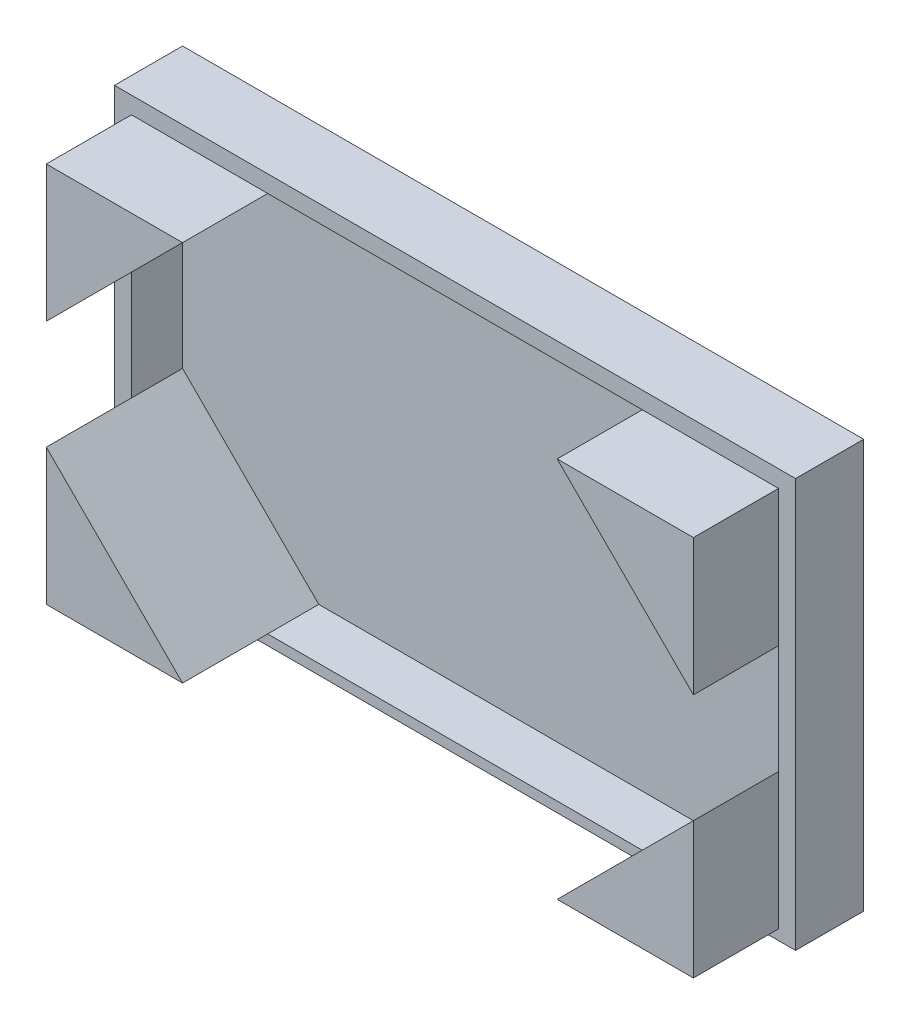
ISO-10303-21;
HEADER;
FILE_DESCRIPTION(('STEP AP214'),'2;1');
FILE_NAME('part.step','',(''),(''),'','','');
FILE_SCHEMA(('AUTOMOTIVE_DESIGN { 1 0 10303 214 1 1 1 1 }'));
ENDSEC;
DATA;
#1=APPLICATION_CONTEXT('core data for automotive mechanical design processes');
#2=APPLICATION_PROTOCOL_DEFINITION('international standard','automotive_design',2000,#1);
#3=PRODUCT_CONTEXT('',#1,'mechanical');
#4=PRODUCT('Part','Part','',(#3));
#5=PRODUCT_RELATED_PRODUCT_CATEGORY('part','',(#4));
#6=PRODUCT_DEFINITION_FORMATION('','',#4);
#7=PRODUCT_DEFINITION_CONTEXT('part definition',#1,'design');
#8=PRODUCT_DEFINITION('design','',#6,#7);
#9=PRODUCT_DEFINITION_SHAPE('','',#8);
#10=(LENGTH_UNIT() NAMED_UNIT(*) SI_UNIT(.MILLI.,.METRE.));
#11=(NAMED_UNIT(*) PLANE_ANGLE_UNIT() SI_UNIT($,.RADIAN.));
#12=(NAMED_UNIT(*) SI_UNIT($,.STERADIAN.) SOLID_ANGLE_UNIT());
#13=UNCERTAINTY_MEASURE_WITH_UNIT(LENGTH_MEASURE(1.E-05),#10,'distance_accuracy_value','');
#14=(GEOMETRIC_REPRESENTATION_CONTEXT(3) GLOBAL_UNCERTAINTY_ASSIGNED_CONTEXT((#13)) GLOBAL_UNIT_ASSIGNED_CONTEXT((#10,
#11,#12)) REPRESENTATION_CONTEXT('',''));
#15=CARTESIAN_POINT('',(0.,0.,0.));
#16=DIRECTION('',(0.,0.,1.));
#17=DIRECTION('',(1.,0.,0.));
#18=AXIS2_PLACEMENT_3D('',#15,#16,#17);
#19=CARTESIAN_POINT('',(0.,0.,2.5));
#20=DIRECTION('',(0.,0.,-1.));
#21=DIRECTION('',(-1.,0.,0.));
#22=AXIS2_PLACEMENT_3D('',#19,#20,#21);
#23=PLANE('',#22);
#24=DIRECTION('',(-0.707106781186548,-0.707106781186547,0.));
#25=VECTOR('',#24,1.);
#26=CARTESIAN_POINT('',(97.5,21.5,2.5));
#27=LINE('',#26,#25);
#28=CARTESIAN_POINT('',(97.5,21.5,2.5));
#29=VERTEX_POINT('',#28);
#30=CARTESIAN_POINT('',(77.5,1.50000000000002,2.5));
#31=VERTEX_POINT('',#30);
#32=EDGE_CURVE('E58',#29,#31,#27,.T.);
#33=ORIENTED_EDGE('',*,*,#32,.F.);
#34=DIRECTION('',(0.,1.,0.));
#35=VECTOR('',#34,1.);
#36=CARTESIAN_POINT('',(97.5,57.5,2.5));
#37=LINE('',#36,#35);
#38=CARTESIAN_POINT('',(97.5,37.5,2.5));
#39=VERTEX_POINT('',#38);
#40=EDGE_CURVE('E277',#29,#39,#37,.T.);
#41=ORIENTED_EDGE('',*,*,#40,.T.);
#42=DIRECTION('',(0.707106781186548,-0.707106781186547,0.));
#43=VECTOR('',#42,1.);
#44=CARTESIAN_POINT('',(97.5,37.5,2.5));
#45=LINE('',#44,#43);
#46=CARTESIAN_POINT('',(77.5,57.5,2.5));
#47=VERTEX_POINT('',#46);
#48=EDGE_CURVE('E206',#47,#39,#45,.T.);
#49=ORIENTED_EDGE('',*,*,#48,.F.);
#50=DIRECTION('',(-1.,0.,0.));
#51=VECTOR('',#50,1.);
#52=CARTESIAN_POINT('',(2.5,57.5,2.5));
#53=LINE('',#52,#51);
#54=CARTESIAN_POINT('',(22.5,57.5,2.5));
#55=VERTEX_POINT('',#54);
#56=EDGE_CURVE('E294',#47,#55,#53,.T.);
#57=ORIENTED_EDGE('',*,*,#56,.T.);
#58=DIRECTION('',(0.707106781186547,0.707106781186548,0.));
#59=VECTOR('',#58,1.);
#60=CARTESIAN_POINT('',(2.5,37.5,2.5));
#61=LINE('',#60,#59);
#62=CARTESIAN_POINT('',(2.5,37.5,2.5));
#63=VERTEX_POINT('',#62);
#64=EDGE_CURVE('E252',#63,#55,#61,.T.);
#65=ORIENTED_EDGE('',*,*,#64,.F.);
#66=DIRECTION('',(0.,-1.,0.));
#67=VECTOR('',#66,1.);
#68=CARTESIAN_POINT('',(2.5,57.5,2.5));
#69=LINE('',#68,#67);
#70=CARTESIAN_POINT('',(2.5,21.5,2.5));
#71=VERTEX_POINT('',#70);
#72=EDGE_CURVE('E298',#63,#71,#69,.T.);
#73=ORIENTED_EDGE('',*,*,#72,.T.);
#74=DIRECTION('',(-0.707106781186547,0.707106781186548,0.));
#75=VECTOR('',#74,1.);
#76=CARTESIAN_POINT('',(2.5,21.5,2.5));
#77=LINE('',#76,#75);
#78=CARTESIAN_POINT('',(22.5,1.50000000000002,2.5));
#79=VERTEX_POINT('',#78);
#80=EDGE_CURVE('E233',#79,#71,#77,.T.);
#81=ORIENTED_EDGE('',*,*,#80,.F.);
#82=DIRECTION('',(1.,0.,0.));
#83=VECTOR('',#82,1.);
#84=CARTESIAN_POINT('',(2.50000000000001,1.50000000000002,2.5));
#85=LINE('',#84,#83);
#86=EDGE_CURVE('E300',#79,#31,#85,.T.);
#87=ORIENTED_EDGE('',*,*,#86,.T.);
#88=EDGE_LOOP('',(#33,#41,#49,#57,#65,#73,#81,#87));
#89=FACE_BOUND('',#88,.T.);
#90=ADVANCED_FACE('F44',(#89),#23,.F.);
#91=CARTESIAN_POINT('',(97.5,57.5,10.));
#92=DIRECTION('',(-1.,0.,0.));
#93=DIRECTION('',(0.,-1.,0.));
#94=AXIS2_PLACEMENT_3D('',#91,#92,#93);
#95=PLANE('',#94);
#96=ORIENTED_EDGE('',*,*,#40,.F.);
#97=DIRECTION('',(0.,0.,-1.));
#98=VECTOR('',#97,1.);
#99=CARTESIAN_POINT('',(97.5,21.5,22.5));
#100=LINE('',#99,#98);
#101=CARTESIAN_POINT('',(97.5,21.5,10.));
#102=VERTEX_POINT('',#101);
#103=EDGE_CURVE('E210',#102,#29,#100,.T.);
#104=ORIENTED_EDGE('',*,*,#103,.F.);
#105=DIRECTION('',(0.,1.,0.));
#106=VECTOR('',#105,1.);
#107=CARTESIAN_POINT('',(97.5,57.5,10.));
#108=LINE('',#107,#106);
#109=CARTESIAN_POINT('',(97.5,37.5,10.));
#110=VERTEX_POINT('',#109);
#111=EDGE_CURVE('E276',#102,#110,#108,.T.);
#112=ORIENTED_EDGE('',*,*,#111,.T.);
#113=DIRECTION('',(0.,0.,-1.));
#114=VECTOR('',#113,1.);
#115=CARTESIAN_POINT('',(97.5,37.5,10.));
#116=LINE('',#115,#114);
#117=EDGE_CURVE('E11',#110,#39,#116,.T.);
#118=ORIENTED_EDGE('',*,*,#117,.T.);
#119=EDGE_LOOP('',(#96,#104,#112,#118));
#120=FACE_BOUND('',#119,.T.);
#121=ADVANCED_FACE('F349',(#120),#95,.T.);
#122=CARTESIAN_POINT('',(2.50000000000001,1.50000000000002,10.));
#123=DIRECTION('',(0.,1.,0.));
#124=DIRECTION('',(-1.,0.,0.));
#125=AXIS2_PLACEMENT_3D('',#122,#123,#124);
#126=PLANE('',#125);
#127=DIRECTION('',(1.,0.,0.));
#128=VECTOR('',#127,1.);
#129=CARTESIAN_POINT('',(2.50000000000001,1.50000000000002,10.));
#130=LINE('',#129,#128);
#131=CARTESIAN_POINT('',(22.5,1.50000000000002,10.));
#132=VERTEX_POINT('',#131);
#133=CARTESIAN_POINT('',(77.5,1.50000000000002,10.));
#134=VERTEX_POINT('',#133);
#135=EDGE_CURVE('E295',#132,#134,#130,.T.);
#136=ORIENTED_EDGE('',*,*,#135,.T.);
#137=DIRECTION('',(0.,0.,-1.));
#138=VECTOR('',#137,1.);
#139=CARTESIAN_POINT('',(77.5,1.50000000000002,22.5));
#140=LINE('',#139,#138);
#141=EDGE_CURVE('E66',#134,#31,#140,.T.);
#142=ORIENTED_EDGE('',*,*,#141,.T.);
#143=ORIENTED_EDGE('',*,*,#86,.F.);
#144=DIRECTION('',(0.,0.,1.));
#145=VECTOR('',#144,1.);
#146=CARTESIAN_POINT('',(22.5,1.50000000000002,10.));
#147=LINE('',#146,#145);
#148=EDGE_CURVE('E52',#79,#132,#147,.T.);
#149=ORIENTED_EDGE('',*,*,#148,.T.);
#150=EDGE_LOOP('',(#136,#142,#143,#149));
#151=FACE_BOUND('',#150,.T.);
#152=ADVANCED_FACE('F331',(#151),#126,.T.);
#153=CARTESIAN_POINT('',(2.5,57.5,10.));
#154=DIRECTION('',(0.,-1.,0.));
#155=DIRECTION('',(0.,0.,-1.));
#156=AXIS2_PLACEMENT_3D('',#153,#154,#155);
#157=PLANE('',#156);
#158=ORIENTED_EDGE('',*,*,#56,.F.);
#159=DIRECTION('',(0.,0.,-1.));
#160=VECTOR('',#159,1.);
#161=CARTESIAN_POINT('',(77.5,57.5,22.5));
#162=LINE('',#161,#160);
#163=CARTESIAN_POINT('',(77.5,57.5,10.));
#164=VERTEX_POINT('',#163);
#165=EDGE_CURVE('E221',#164,#47,#162,.T.);
#166=ORIENTED_EDGE('',*,*,#165,.F.);
#167=DIRECTION('',(-1.,0.,0.));
#168=VECTOR('',#167,1.);
#169=CARTESIAN_POINT('',(2.5,57.5,10.));
#170=LINE('',#169,#168);
#171=CARTESIAN_POINT('',(22.5,57.5,10.));
#172=VERTEX_POINT('',#171);
#173=EDGE_CURVE('E279',#164,#172,#170,.T.);
#174=ORIENTED_EDGE('',*,*,#173,.T.);
#175=DIRECTION('',(0.,0.,-1.));
#176=VECTOR('',#175,1.);
#177=CARTESIAN_POINT('',(22.5,57.5,22.5));
#178=LINE('',#177,#176);
#179=EDGE_CURVE('E264',#172,#55,#178,.T.);
#180=ORIENTED_EDGE('',*,*,#179,.T.);
#181=EDGE_LOOP('',(#158,#166,#174,#180));
#182=FACE_BOUND('',#181,.T.);
#183=ADVANCED_FACE('F370',(#182),#157,.T.);
#184=CARTESIAN_POINT('',(2.5,57.5,10.));
#185=DIRECTION('',(1.,0.,0.));
#186=DIRECTION('',(0.,1.,0.));
#187=AXIS2_PLACEMENT_3D('',#184,#185,#186);
#188=PLANE('',#187);
#189=DIRECTION('',(0.,-1.,0.));
#190=VECTOR('',#189,1.);
#191=CARTESIAN_POINT('',(2.5,57.5,10.));
#192=LINE('',#191,#190);
#193=CARTESIAN_POINT('',(2.5,37.5,10.));
#194=VERTEX_POINT('',#193);
#195=CARTESIAN_POINT('',(2.5,21.5,10.));
#196=VERTEX_POINT('',#195);
#197=EDGE_CURVE('E282',#194,#196,#192,.T.);
#198=ORIENTED_EDGE('',*,*,#197,.T.);
#199=DIRECTION('',(0.,0.,-1.));
#200=VECTOR('',#199,1.);
#201=CARTESIAN_POINT('',(2.5,21.5,22.5));
#202=LINE('',#201,#200);
#203=EDGE_CURVE('E239',#196,#71,#202,.T.);
#204=ORIENTED_EDGE('',*,*,#203,.T.);
#205=ORIENTED_EDGE('',*,*,#72,.F.);
#206=DIRECTION('',(0.,0.,-1.));
#207=VECTOR('',#206,1.);
#208=CARTESIAN_POINT('',(2.5,37.5,22.5));
#209=LINE('',#208,#207);
#210=EDGE_CURVE('E267',#194,#63,#209,.T.);
#211=ORIENTED_EDGE('',*,*,#210,.F.);
#212=EDGE_LOOP('',(#198,#204,#205,#211));
#213=FACE_BOUND('',#212,.T.);
#214=ADVANCED_FACE('F378',(#213),#188,.T.);
#215=CARTESIAN_POINT('',(0.,0.,2.5));
#216=DIRECTION('',(1.,0.,0.));
#217=DIRECTION('',(0.,0.,-1.));
#218=AXIS2_PLACEMENT_3D('',#215,#216,#217);
#219=PLANE('',#218);
#220=DIRECTION('',(0.,-1.,0.));
#221=VECTOR('',#220,1.);
#222=CARTESIAN_POINT('',(0.,0.,0.));
#223=LINE('',#222,#221);
#224=CARTESIAN_POINT('',(0.,60.,0.));
#225=VERTEX_POINT('',#224);
#226=CARTESIAN_POINT('',(0.,0.,0.));
#227=VERTEX_POINT('',#226);
#228=EDGE_CURVE('E315',#225,#227,#223,.T.);
#229=ORIENTED_EDGE('',*,*,#228,.T.);
#230=DIRECTION('',(0.,0.,-1.));
#231=VECTOR('',#230,1.);
#232=CARTESIAN_POINT('',(0.,0.,2.5));
#233=LINE('',#232,#231);
#234=CARTESIAN_POINT('',(0.,0.,10.));
#235=VERTEX_POINT('',#234);
#236=EDGE_CURVE('E329',#235,#227,#233,.T.);
#237=ORIENTED_EDGE('',*,*,#236,.F.);
#238=DIRECTION('',(0.,-1.,0.));
#239=VECTOR('',#238,1.);
#240=CARTESIAN_POINT('',(0.,60.,10.));
#241=LINE('',#240,#239);
#242=CARTESIAN_POINT('',(0.,60.,10.));
#243=VERTEX_POINT('',#242);
#244=EDGE_CURVE('E308',#243,#235,#241,.T.);
#245=ORIENTED_EDGE('',*,*,#244,.F.);
#246=DIRECTION('',(0.,0.,-1.));
#247=VECTOR('',#246,1.);
#248=CARTESIAN_POINT('',(0.,60.,2.5));
#249=LINE('',#248,#247);
#250=EDGE_CURVE('E321',#243,#225,#249,.T.);
#251=ORIENTED_EDGE('',*,*,#250,.T.);
#252=EDGE_LOOP('',(#229,#237,#245,#251));
#253=FACE_BOUND('',#252,.T.);
#254=ADVANCED_FACE('F50',(#253),#219,.F.);
#255=CARTESIAN_POINT('',(0.,0.,2.5));
#256=DIRECTION('',(0.,1.,0.));
#257=DIRECTION('',(0.,0.,1.));
#258=AXIS2_PLACEMENT_3D('',#255,#256,#257);
#259=PLANE('',#258);
#260=DIRECTION('',(1.,0.,0.));
#261=VECTOR('',#260,1.);
#262=CARTESIAN_POINT('',(0.,0.,0.));
#263=LINE('',#262,#261);
#264=CARTESIAN_POINT('',(100.,0.,0.));
#265=VERTEX_POINT('',#264);
#266=EDGE_CURVE('E312',#227,#265,#263,.T.);
#267=ORIENTED_EDGE('',*,*,#266,.T.);
#268=DIRECTION('',(0.,0.,-1.));
#269=VECTOR('',#268,1.);
#270=CARTESIAN_POINT('',(100.,0.,2.5));
#271=LINE('',#270,#269);
#272=CARTESIAN_POINT('',(100.,0.,10.));
#273=VERTEX_POINT('',#272);
#274=EDGE_CURVE('E330',#273,#265,#271,.T.);
#275=ORIENTED_EDGE('',*,*,#274,.F.);
#276=DIRECTION('',(1.,0.,0.));
#277=VECTOR('',#276,1.);
#278=CARTESIAN_POINT('',(0.,0.,10.));
#279=LINE('',#278,#277);
#280=EDGE_CURVE('E310',#235,#273,#279,.T.);
#281=ORIENTED_EDGE('',*,*,#280,.F.);
#282=ORIENTED_EDGE('',*,*,#236,.T.);
#283=EDGE_LOOP('',(#267,#275,#281,#282));
#284=FACE_BOUND('',#283,.T.);
#285=ADVANCED_FACE('F423',(#284),#259,.F.);
#286=CARTESIAN_POINT('',(100.,0.,2.5));
#287=DIRECTION('',(-1.,0.,0.));
#288=DIRECTION('',(0.,0.,1.));
#289=AXIS2_PLACEMENT_3D('',#286,#287,#288);
#290=PLANE('',#289);
#291=DIRECTION('',(0.,1.,0.));
#292=VECTOR('',#291,1.);
#293=CARTESIAN_POINT('',(100.,0.,0.));
#294=LINE('',#293,#292);
#295=CARTESIAN_POINT('',(100.,60.,0.));
#296=VERTEX_POINT('',#295);
#297=EDGE_CURVE('E320',#265,#296,#294,.T.);
#298=ORIENTED_EDGE('',*,*,#297,.T.);
#299=DIRECTION('',(0.,0.,-1.));
#300=VECTOR('',#299,1.);
#301=CARTESIAN_POINT('',(100.,60.,2.5));
#302=LINE('',#301,#300);
#303=CARTESIAN_POINT('',(100.,60.,10.));
#304=VERTEX_POINT('',#303);
#305=EDGE_CURVE('E322',#304,#296,#302,.T.);
#306=ORIENTED_EDGE('',*,*,#305,.F.);
#307=DIRECTION('',(0.,1.,0.));
#308=VECTOR('',#307,1.);
#309=CARTESIAN_POINT('',(100.,60.,10.));
#310=LINE('',#309,#308);
#311=EDGE_CURVE('E292',#273,#304,#310,.T.);
#312=ORIENTED_EDGE('',*,*,#311,.F.);
#313=ORIENTED_EDGE('',*,*,#274,.T.);
#314=EDGE_LOOP('',(#298,#306,#312,#313));
#315=FACE_BOUND('',#314,.T.);
#316=ADVANCED_FACE('F416',(#315),#290,.F.);
#317=CARTESIAN_POINT('',(0.,60.,2.5));
#318=DIRECTION('',(0.,-1.,0.));
#319=DIRECTION('',(0.,0.,-1.));
#320=AXIS2_PLACEMENT_3D('',#317,#318,#319);
#321=PLANE('',#320);
#322=DIRECTION('',(-1.,0.,0.));
#323=VECTOR('',#322,1.);
#324=CARTESIAN_POINT('',(0.,60.,0.));
#325=LINE('',#324,#323);
#326=EDGE_CURVE('E317',#296,#225,#325,.T.);
#327=ORIENTED_EDGE('',*,*,#326,.T.);
#328=ORIENTED_EDGE('',*,*,#250,.F.);
#329=DIRECTION('',(-1.,0.,0.));
#330=VECTOR('',#329,1.);
#331=CARTESIAN_POINT('',(0.,60.,10.));
#332=LINE('',#331,#330);
#333=EDGE_CURVE('E301',#304,#243,#332,.T.);
#334=ORIENTED_EDGE('',*,*,#333,.F.);
#335=ORIENTED_EDGE('',*,*,#305,.T.);
#336=EDGE_LOOP('',(#327,#328,#334,#335));
#337=FACE_BOUND('',#336,.T.);
#338=ADVANCED_FACE('F414',(#337),#321,.F.);
#339=CARTESIAN_POINT('',(0.,0.,0.));
#340=DIRECTION('',(0.,0.,-1.));
#341=DIRECTION('',(-1.,0.,0.));
#342=AXIS2_PLACEMENT_3D('',#339,#340,#341);
#343=PLANE('',#342);
#344=ORIENTED_EDGE('',*,*,#228,.F.);
#345=ORIENTED_EDGE('',*,*,#326,.F.);
#346=ORIENTED_EDGE('',*,*,#297,.F.);
#347=ORIENTED_EDGE('',*,*,#266,.F.);
#348=EDGE_LOOP('',(#344,#345,#346,#347));
#349=FACE_BOUND('',#348,.T.);
#350=ADVANCED_FACE('F413',(#349),#343,.T.);
#351=CARTESIAN_POINT('',(0.,0.,10.));
#352=DIRECTION('',(0.,0.,1.));
#353=DIRECTION('',(1.,0.,0.));
#354=AXIS2_PLACEMENT_3D('',#351,#352,#353);
#355=PLANE('',#354);
#356=ORIENTED_EDGE('',*,*,#311,.T.);
#357=ORIENTED_EDGE('',*,*,#333,.T.);
#358=ORIENTED_EDGE('',*,*,#244,.T.);
#359=ORIENTED_EDGE('',*,*,#280,.T.);
#360=EDGE_LOOP('',(#356,#357,#358,#359));
#361=FACE_BOUND('',#360,.T.);
#362=CARTESIAN_POINT('',(97.5,57.5,10.));
#363=VERTEX_POINT('',#362);
#364=EDGE_CURVE('E283',#363,#164,#170,.T.);
#365=ORIENTED_EDGE('',*,*,#364,.F.);
#366=EDGE_CURVE('E278',#110,#363,#108,.T.);
#367=ORIENTED_EDGE('',*,*,#366,.F.);
#368=ORIENTED_EDGE('',*,*,#111,.F.);
#369=CARTESIAN_POINT('',(97.5,1.50000000000002,10.));
#370=VERTEX_POINT('',#369);
#371=EDGE_CURVE('E202',#370,#102,#108,.T.);
#372=ORIENTED_EDGE('',*,*,#371,.F.);
#373=EDGE_CURVE('E290',#134,#370,#130,.T.);
#374=ORIENTED_EDGE('',*,*,#373,.F.);
#375=ORIENTED_EDGE('',*,*,#135,.F.);
#376=CARTESIAN_POINT('',(2.5,1.50000000000002,10.));
#377=VERTEX_POINT('',#376);
#378=EDGE_CURVE('E286',#377,#132,#130,.T.);
#379=ORIENTED_EDGE('',*,*,#378,.F.);
#380=DIRECTION('',(0.,1.,0.));
#381=VECTOR('',#380,1.);
#382=CARTESIAN_POINT('',(2.5,0.,10.));
#383=LINE('',#382,#381);
#384=EDGE_CURVE('E249',#377,#196,#383,.T.);
#385=ORIENTED_EDGE('',*,*,#384,.T.);
#386=ORIENTED_EDGE('',*,*,#197,.F.);
#387=CARTESIAN_POINT('',(2.5,57.5,10.));
#388=VERTEX_POINT('',#387);
#389=EDGE_CURVE('E285',#388,#194,#192,.T.);
#390=ORIENTED_EDGE('',*,*,#389,.F.);
#391=DIRECTION('',(1.,0.,0.));
#392=VECTOR('',#391,1.);
#393=CARTESIAN_POINT('',(0.,57.5,10.));
#394=LINE('',#393,#392);
#395=EDGE_CURVE('E272',#388,#172,#394,.T.);
#396=ORIENTED_EDGE('',*,*,#395,.T.);
#397=ORIENTED_EDGE('',*,*,#173,.F.);
#398=EDGE_LOOP('',(#365,#367,#368,#372,#374,#375,#379,#385,#386,#390,#396,#397));
#399=FACE_BOUND('',#398,.T.);
#400=ADVANCED_FACE('F336',(#361,#399),#355,.T.);
#401=CARTESIAN_POINT('',(2.5,57.5,22.5));
#402=DIRECTION('',(1.,0.,0.));
#403=DIRECTION('',(0.,1.,0.));
#404=AXIS2_PLACEMENT_3D('',#401,#402,#403);
#405=PLANE('',#404);
#406=ORIENTED_EDGE('',*,*,#389,.T.);
#407=CARTESIAN_POINT('',(2.5,37.5,22.5));
#408=VERTEX_POINT('',#407);
#409=EDGE_CURVE('E269',#408,#194,#209,.T.);
#410=ORIENTED_EDGE('',*,*,#409,.F.);
#411=DIRECTION('',(0.,-1.,0.));
#412=VECTOR('',#411,1.);
#413=CARTESIAN_POINT('',(2.5,57.5,22.5));
#414=LINE('',#413,#412);
#415=CARTESIAN_POINT('',(2.5,57.5,22.5));
#416=VERTEX_POINT('',#415);
#417=EDGE_CURVE('E251',#416,#408,#414,.T.);
#418=ORIENTED_EDGE('',*,*,#417,.F.);
#419=DIRECTION('',(0.,0.,-1.));
#420=VECTOR('',#419,1.);
#421=CARTESIAN_POINT('',(2.5,57.5,22.5));
#422=LINE('',#421,#420);
#423=EDGE_CURVE('E257',#416,#388,#422,.T.);
#424=ORIENTED_EDGE('',*,*,#423,.T.);
#425=EDGE_LOOP('',(#406,#410,#418,#424));
#426=FACE_BOUND('',#425,.T.);
#427=ADVANCED_FACE('F384',(#426),#405,.F.);
#428=CARTESIAN_POINT('',(2.5,37.5,22.5));
#429=DIRECTION('',(-0.707106781186548,0.707106781186547,0.));
#430=DIRECTION('',(-0.707106781186547,-0.707106781186548,0.));
#431=AXIS2_PLACEMENT_3D('',#428,#429,#430);
#432=PLANE('',#431);
#433=ORIENTED_EDGE('',*,*,#64,.T.);
#434=ORIENTED_EDGE('',*,*,#179,.F.);
#435=CARTESIAN_POINT('',(22.5,57.5,22.5));
#436=VERTEX_POINT('',#435);
#437=EDGE_CURVE('E266',#436,#172,#178,.T.);
#438=ORIENTED_EDGE('',*,*,#437,.F.);
#439=DIRECTION('',(0.707106781186547,0.707106781186548,0.));
#440=VECTOR('',#439,1.);
#441=CARTESIAN_POINT('',(2.5,37.5,22.5));
#442=LINE('',#441,#440);
#443=EDGE_CURVE('E258',#408,#436,#442,.T.);
#444=ORIENTED_EDGE('',*,*,#443,.F.);
#445=ORIENTED_EDGE('',*,*,#409,.T.);
#446=ORIENTED_EDGE('',*,*,#210,.T.);
#447=EDGE_LOOP('',(#433,#434,#438,#444,#445,#446));
#448=FACE_BOUND('',#447,.T.);
#449=ADVANCED_FACE('F379',(#448),#432,.F.);
#450=CARTESIAN_POINT('',(2.5,57.5,22.5));
#451=DIRECTION('',(0.,-1.,0.));
#452=DIRECTION('',(0.,0.,-1.));
#453=AXIS2_PLACEMENT_3D('',#450,#451,#452);
#454=PLANE('',#453);
#455=ORIENTED_EDGE('',*,*,#395,.F.);
#456=ORIENTED_EDGE('',*,*,#423,.F.);
#457=DIRECTION('',(-1.,0.,0.));
#458=VECTOR('',#457,1.);
#459=CARTESIAN_POINT('',(2.5,57.5,22.5));
#460=LINE('',#459,#458);
#461=EDGE_CURVE('E256',#436,#416,#460,.T.);
#462=ORIENTED_EDGE('',*,*,#461,.F.);
#463=ORIENTED_EDGE('',*,*,#437,.T.);
#464=EDGE_LOOP('',(#455,#456,#462,#463));
#465=FACE_BOUND('',#464,.T.);
#466=ADVANCED_FACE('F389',(#465),#454,.F.);
#467=CARTESIAN_POINT('',(0.,0.,22.5));
#468=DIRECTION('',(0.,0.,1.));
#469=DIRECTION('',(1.,0.,0.));
#470=AXIS2_PLACEMENT_3D('',#467,#468,#469);
#471=PLANE('',#470);
#472=ORIENTED_EDGE('',*,*,#417,.T.);
#473=ORIENTED_EDGE('',*,*,#443,.T.);
#474=ORIENTED_EDGE('',*,*,#461,.T.);
#475=EDGE_LOOP('',(#472,#473,#474));
#476=FACE_BOUND('',#475,.T.);
#477=ADVANCED_FACE('F393',(#476),#471,.T.);
#478=CARTESIAN_POINT('',(2.5,1.50000000000002,22.5));
#479=DIRECTION('',(1.,0.,0.));
#480=DIRECTION('',(0.,1.,0.));
#481=AXIS2_PLACEMENT_3D('',#478,#479,#480);
#482=PLANE('',#481);
#483=ORIENTED_EDGE('',*,*,#384,.F.);
#484=DIRECTION('',(0.,0.,-1.));
#485=VECTOR('',#484,1.);
#486=CARTESIAN_POINT('',(2.5,1.50000000000002,22.5));
#487=LINE('',#486,#485);
#488=CARTESIAN_POINT('',(2.5,1.50000000000002,22.5));
#489=VERTEX_POINT('',#488);
#490=EDGE_CURVE('E248',#489,#377,#487,.T.);
#491=ORIENTED_EDGE('',*,*,#490,.F.);
#492=DIRECTION('',(0.,-1.,0.));
#493=VECTOR('',#492,1.);
#494=CARTESIAN_POINT('',(2.5,1.50000000000002,22.5));
#495=LINE('',#494,#493);
#496=CARTESIAN_POINT('',(2.5,21.5,22.5));
#497=VERTEX_POINT('',#496);
#498=EDGE_CURVE('E235',#497,#489,#495,.T.);
#499=ORIENTED_EDGE('',*,*,#498,.F.);
#500=EDGE_CURVE('E243',#497,#196,#202,.T.);
#501=ORIENTED_EDGE('',*,*,#500,.T.);
#502=EDGE_LOOP('',(#483,#491,#499,#501));
#503=FACE_BOUND('',#502,.T.);
#504=ADVANCED_FACE('F392',(#503),#482,.F.);
#505=CARTESIAN_POINT('',(2.5,1.50000000000002,22.5));
#506=DIRECTION('',(0.,1.,0.));
#507=DIRECTION('',(0.,0.,1.));
#508=AXIS2_PLACEMENT_3D('',#505,#506,#507);
#509=PLANE('',#508);
#510=ORIENTED_EDGE('',*,*,#378,.T.);
#511=DIRECTION('',(0.,0.,-1.));
#512=VECTOR('',#511,1.);
#513=CARTESIAN_POINT('',(22.5,1.50000000000002,22.5));
#514=LINE('',#513,#512);
#515=CARTESIAN_POINT('',(22.5,1.50000000000002,22.5));
#516=VERTEX_POINT('',#515);
#517=EDGE_CURVE('E245',#516,#132,#514,.T.);
#518=ORIENTED_EDGE('',*,*,#517,.F.);
#519=DIRECTION('',(1.,0.,0.));
#520=VECTOR('',#519,1.);
#521=CARTESIAN_POINT('',(2.5,1.50000000000002,22.5));
#522=LINE('',#521,#520);
#523=EDGE_CURVE('E232',#489,#516,#522,.T.);
#524=ORIENTED_EDGE('',*,*,#523,.F.);
#525=ORIENTED_EDGE('',*,*,#490,.T.);
#526=EDGE_LOOP('',(#510,#518,#524,#525));
#527=FACE_BOUND('',#526,.T.);
#528=ADVANCED_FACE('F399',(#527),#509,.F.);
#529=CARTESIAN_POINT('',(2.5,21.5,22.5));
#530=DIRECTION('',(-0.707106781186548,-0.707106781186547,0.));
#531=DIRECTION('',(0.707106781186547,-0.707106781186548,0.));
#532=AXIS2_PLACEMENT_3D('',#529,#530,#531);
#533=PLANE('',#532);
#534=ORIENTED_EDGE('',*,*,#80,.T.);
#535=ORIENTED_EDGE('',*,*,#203,.F.);
#536=ORIENTED_EDGE('',*,*,#500,.F.);
#537=DIRECTION('',(-0.707106781186547,0.707106781186548,0.));
#538=VECTOR('',#537,1.);
#539=CARTESIAN_POINT('',(2.5,21.5,22.5));
#540=LINE('',#539,#538);
#541=EDGE_CURVE('E240',#516,#497,#540,.T.);
#542=ORIENTED_EDGE('',*,*,#541,.F.);
#543=ORIENTED_EDGE('',*,*,#517,.T.);
#544=ORIENTED_EDGE('',*,*,#148,.F.);
#545=EDGE_LOOP('',(#534,#535,#536,#542,#543,#544));
#546=FACE_BOUND('',#545,.T.);
#547=ADVANCED_FACE('F521',(#546),#533,.F.);
#548=CARTESIAN_POINT('',(0.,0.,22.5));
#549=DIRECTION('',(0.,0.,-1.));
#550=DIRECTION('',(-1.,0.,0.));
#551=AXIS2_PLACEMENT_3D('',#548,#549,#550);
#552=PLANE('',#551);
#553=ORIENTED_EDGE('',*,*,#498,.T.);
#554=ORIENTED_EDGE('',*,*,#523,.T.);
#555=ORIENTED_EDGE('',*,*,#541,.T.);
#556=EDGE_LOOP('',(#553,#554,#555));
#557=FACE_BOUND('',#556,.T.);
#558=ADVANCED_FACE('F531',(#557),#552,.F.);
#559=CARTESIAN_POINT('',(97.5,57.5,22.5));
#560=DIRECTION('',(-1.,0.,0.));
#561=DIRECTION('',(0.,0.,1.));
#562=AXIS2_PLACEMENT_3D('',#559,#560,#561);
#563=PLANE('',#562);
#564=ORIENTED_EDGE('',*,*,#366,.T.);
#565=DIRECTION('',(0.,0.,-1.));
#566=VECTOR('',#565,1.);
#567=CARTESIAN_POINT('',(97.5,57.5,22.5));
#568=LINE('',#567,#566);
#569=CARTESIAN_POINT('',(97.5,57.5,22.5));
#570=VERTEX_POINT('',#569);
#571=EDGE_CURVE('E227',#570,#363,#568,.T.);
#572=ORIENTED_EDGE('',*,*,#571,.F.);
#573=DIRECTION('',(0.,1.,0.));
#574=VECTOR('',#573,1.);
#575=CARTESIAN_POINT('',(97.5,57.5,22.5));
#576=LINE('',#575,#574);
#577=CARTESIAN_POINT('',(97.5,37.5,22.5));
#578=VERTEX_POINT('',#577);
#579=EDGE_CURVE('E209',#578,#570,#576,.T.);
#580=ORIENTED_EDGE('',*,*,#579,.F.);
#581=DIRECTION('',(0.,0.,-1.));
#582=VECTOR('',#581,1.);
#583=CARTESIAN_POINT('',(97.5,37.5,22.5));
#584=LINE('',#583,#582);
#585=EDGE_CURVE('E219',#578,#110,#584,.T.);
#586=ORIENTED_EDGE('',*,*,#585,.T.);
#587=EDGE_LOOP('',(#564,#572,#580,#586));
#588=FACE_BOUND('',#587,.T.);
#589=ADVANCED_FACE('F355',(#588),#563,.F.);
#590=CARTESIAN_POINT('',(97.5,57.5,22.5));
#591=DIRECTION('',(0.,-1.,0.));
#592=DIRECTION('',(0.,0.,-1.));
#593=AXIS2_PLACEMENT_3D('',#590,#591,#592);
#594=PLANE('',#593);
#595=ORIENTED_EDGE('',*,*,#364,.T.);
#596=CARTESIAN_POINT('',(77.5,57.5,22.5));
#597=VERTEX_POINT('',#596);
#598=EDGE_CURVE('E223',#597,#164,#162,.T.);
#599=ORIENTED_EDGE('',*,*,#598,.F.);
#600=DIRECTION('',(-1.,0.,0.));
#601=VECTOR('',#600,1.);
#602=CARTESIAN_POINT('',(97.5,57.5,22.5));
#603=LINE('',#602,#601);
#604=EDGE_CURVE('E220',#570,#597,#603,.T.);
#605=ORIENTED_EDGE('',*,*,#604,.F.);
#606=ORIENTED_EDGE('',*,*,#571,.T.);
#607=EDGE_LOOP('',(#595,#599,#605,#606));
#608=FACE_BOUND('',#607,.T.);
#609=ADVANCED_FACE('F356',(#608),#594,.F.);
#610=CARTESIAN_POINT('',(97.5,37.5,22.5));
#611=DIRECTION('',(0.707106781186547,0.707106781186548,0.));
#612=DIRECTION('',(-0.707106781186548,0.707106781186547,0.));
#613=AXIS2_PLACEMENT_3D('',#610,#611,#612);
#614=PLANE('',#613);
#615=ORIENTED_EDGE('',*,*,#48,.T.);
#616=ORIENTED_EDGE('',*,*,#117,.F.);
#617=ORIENTED_EDGE('',*,*,#585,.F.);
#618=DIRECTION('',(0.707106781186548,-0.707106781186547,0.));
#619=VECTOR('',#618,1.);
#620=CARTESIAN_POINT('',(97.5,37.5,22.5));
#621=LINE('',#620,#619);
#622=EDGE_CURVE('E218',#597,#578,#621,.T.);
#623=ORIENTED_EDGE('',*,*,#622,.F.);
#624=ORIENTED_EDGE('',*,*,#598,.T.);
#625=ORIENTED_EDGE('',*,*,#165,.T.);
#626=EDGE_LOOP('',(#615,#616,#617,#623,#624,#625));
#627=FACE_BOUND('',#626,.T.);
#628=ADVANCED_FACE('F367',(#627),#614,.F.);
#629=CARTESIAN_POINT('',(0.,0.,22.5));
#630=DIRECTION('',(0.,0.,-1.));
#631=DIRECTION('',(-1.,0.,0.));
#632=AXIS2_PLACEMENT_3D('',#629,#630,#631);
#633=PLANE('',#632);
#634=ORIENTED_EDGE('',*,*,#579,.T.);
#635=ORIENTED_EDGE('',*,*,#604,.T.);
#636=ORIENTED_EDGE('',*,*,#622,.T.);
#637=EDGE_LOOP('',(#634,#635,#636));
#638=FACE_BOUND('',#637,.T.);
#639=ADVANCED_FACE('F567',(#638),#633,.F.);
#640=CARTESIAN_POINT('',(97.5,1.50000000000002,22.5));
#641=DIRECTION('',(-1.,0.,0.));
#642=DIRECTION('',(0.,0.,1.));
#643=AXIS2_PLACEMENT_3D('',#640,#641,#642);
#644=PLANE('',#643);
#645=ORIENTED_EDGE('',*,*,#371,.T.);
#646=CARTESIAN_POINT('',(97.5,21.5,22.5));
#647=VERTEX_POINT('',#646);
#648=EDGE_CURVE('E190',#647,#102,#100,.T.);
#649=ORIENTED_EDGE('',*,*,#648,.F.);
#650=DIRECTION('',(0.,1.,0.));
#651=VECTOR('',#650,1.);
#652=CARTESIAN_POINT('',(97.5,1.50000000000002,22.5));
#653=LINE('',#652,#651);
#654=CARTESIAN_POINT('',(97.5,1.50000000000002,22.5));
#655=VERTEX_POINT('',#654);
#656=EDGE_CURVE('E192',#655,#647,#653,.T.);
#657=ORIENTED_EDGE('',*,*,#656,.F.);
#658=DIRECTION('',(0.,0.,-1.));
#659=VECTOR('',#658,1.);
#660=CARTESIAN_POINT('',(97.5,1.50000000000002,22.5));
#661=LINE('',#660,#659);
#662=EDGE_CURVE('E344',#655,#370,#661,.T.);
#663=ORIENTED_EDGE('',*,*,#662,.T.);
#664=EDGE_LOOP('',(#645,#649,#657,#663));
#665=FACE_BOUND('',#664,.T.);
#666=ADVANCED_FACE('F204',(#665),#644,.F.);
#667=CARTESIAN_POINT('',(97.5,21.5,22.5));
#668=DIRECTION('',(0.707106781186547,-0.707106781186548,0.));
#669=DIRECTION('',(0.707106781186548,0.707106781186547,0.));
#670=AXIS2_PLACEMENT_3D('',#667,#668,#669);
#671=PLANE('',#670);
#672=ORIENTED_EDGE('',*,*,#32,.T.);
#673=ORIENTED_EDGE('',*,*,#141,.F.);
#674=CARTESIAN_POINT('',(77.5,1.50000000000002,22.5));
#675=VERTEX_POINT('',#674);
#676=EDGE_CURVE('E193',#675,#134,#140,.T.);
#677=ORIENTED_EDGE('',*,*,#676,.F.);
#678=DIRECTION('',(-0.707106781186548,-0.707106781186547,0.));
#679=VECTOR('',#678,1.);
#680=CARTESIAN_POINT('',(97.5,21.5,22.5));
#681=LINE('',#680,#679);
#682=EDGE_CURVE('E184',#647,#675,#681,.T.);
#683=ORIENTED_EDGE('',*,*,#682,.F.);
#684=ORIENTED_EDGE('',*,*,#648,.T.);
#685=ORIENTED_EDGE('',*,*,#103,.T.);
#686=EDGE_LOOP('',(#672,#673,#677,#683,#684,#685));
#687=FACE_BOUND('',#686,.T.);
#688=ADVANCED_FACE('F188',(#687),#671,.F.);
#689=CARTESIAN_POINT('',(97.5,1.50000000000002,22.5));
#690=DIRECTION('',(0.,1.,0.));
#691=DIRECTION('',(0.,0.,1.));
#692=AXIS2_PLACEMENT_3D('',#689,#690,#691);
#693=PLANE('',#692);
#694=ORIENTED_EDGE('',*,*,#373,.T.);
#695=ORIENTED_EDGE('',*,*,#662,.F.);
#696=DIRECTION('',(1.,0.,0.));
#697=VECTOR('',#696,1.);
#698=CARTESIAN_POINT('',(97.5,1.50000000000002,22.5));
#699=LINE('',#698,#697);
#700=EDGE_CURVE('E194',#675,#655,#699,.T.);
#701=ORIENTED_EDGE('',*,*,#700,.F.);
#702=ORIENTED_EDGE('',*,*,#676,.T.);
#703=EDGE_LOOP('',(#694,#695,#701,#702));
#704=FACE_BOUND('',#703,.T.);
#705=ADVANCED_FACE('F341',(#704),#693,.F.);
#706=CARTESIAN_POINT('',(0.,0.,22.5));
#707=DIRECTION('',(0.,0.,1.));
#708=DIRECTION('',(1.,0.,0.));
#709=AXIS2_PLACEMENT_3D('',#706,#707,#708);
#710=PLANE('',#709);
#711=ORIENTED_EDGE('',*,*,#656,.T.);
#712=ORIENTED_EDGE('',*,*,#682,.T.);
#713=ORIENTED_EDGE('',*,*,#700,.T.);
#714=EDGE_LOOP('',(#711,#712,#713));
#715=FACE_BOUND('',#714,.T.);
#716=ADVANCED_FACE('F196',(#715),#710,.T.);
#717=CLOSED_SHELL('',(#90,#121,#152,#183,#214,#254,#285,#316,#338,#350,#400,#427,#449,#466,#477,
#504,#528,#547,#558,#589,#609,#628,#639,#666,#688,#705,#716));
#718=MANIFOLD_SOLID_BREP('B2',#717);
#719=ADVANCED_BREP_SHAPE_REPRESENTATION('',(#18,#718),#14);
#720=SHAPE_DEFINITION_REPRESENTATION(#9,#719);
ENDSEC;
END-ISO-10303-21;
